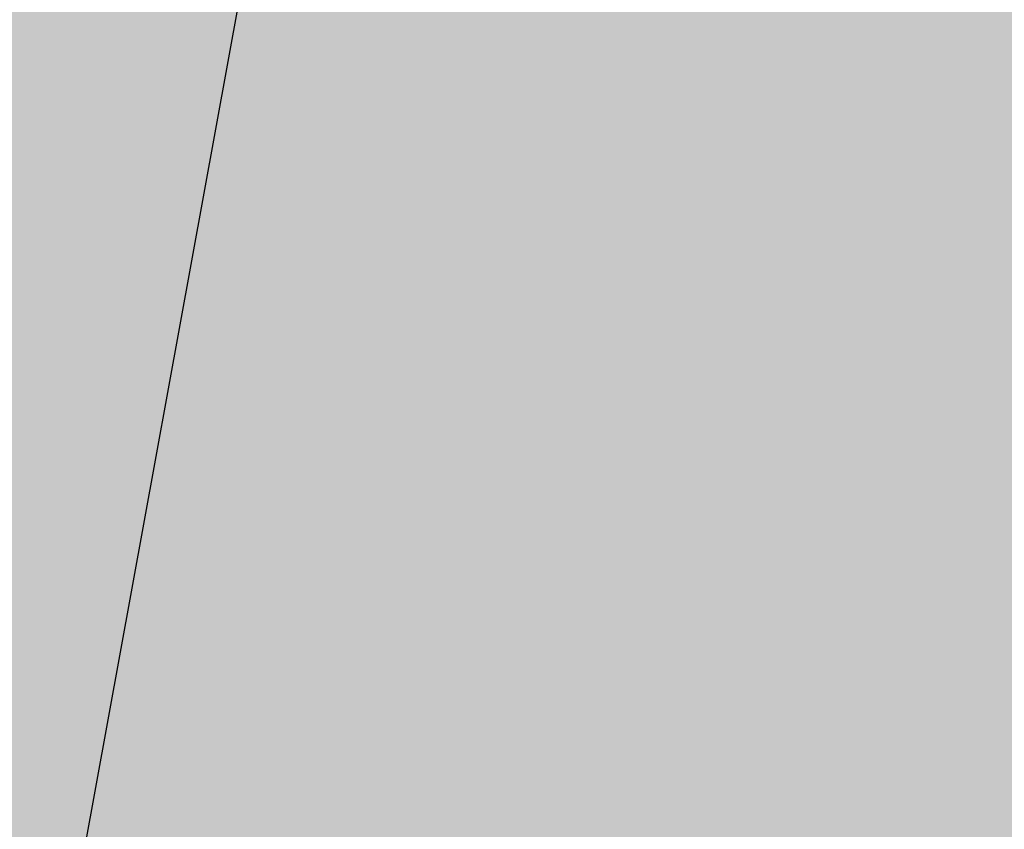
# Model space of a CAD drawing. Units: feet. Extents: x 3168 to 4724, y 827 to 1477.
# Tile 225 of 256: x 3379.08 to 3394.29, y 1074.89 to 1087.4. Entities that reach past the tile are written whole.
import ezdxf

# ---------------------------------------------------------------- set-up
doc = ezdxf.new("R2010")
doc.units = ezdxf.units.FT
doc.layers.add('A-ELEV-PATT', color=8, linetype='Continuous', lineweight=13)
doc.layers.add('C-TOPO', color=3, linetype='Continuous', lineweight=25)

msp = doc.modelspace()

# ---------------------------------------------------------------- hatches: boundary and pattern name
at = {"layer": 'A-ELEV-PATT'}
h = msp.add_hatch(color=256, dxfattribs=at)
h.dxf.hatch_style = 1
edge = h.paths.add_edge_path()
edge.add_ellipse((3552.906, 979.22), major_axis=(36.745, 0), ratio=0.484848, start_angle=0, end_angle=360)
edge = h.paths.add_edge_path()
edge.add_ellipse((3559.892, 929.252), major_axis=(36.745, 0), ratio=0.484848, start_angle=0, end_angle=360)
edge = h.paths.add_edge_path()
edge.add_line((3299.317, 1198.606), (3479.917, 1198.606))
edge.add_line((3479.917, 1198.606), (3479.917, 1209.869))
edge.add_spline(control_points=[(3479.917, 1209.869), (3464.301, 1209.869), (3448.686, 1209.869), (3410.949, 1209.869), (3388.828, 1209.869), (3355.647, 1209.869), (3344.586, 1209.869), (3327.996, 1209.869), (3322.466, 1209.869), (3314.17, 1209.869), (3311.405, 1209.869), (3307.257, 1209.869), (3305.875, 1209.869), (3303.801, 1209.869), (3303.11, 1209.869), (3302.073, 1209.869), (3301.727, 1209.869), (3301.209, 1209.869), (3301.036, 1209.869), (3300.777, 1209.869), (3300.69, 1209.869), (3300.561, 1209.869), (3300.517, 1209.869), (3300.453, 1209.869), (3300.431, 1209.869), (3300.399, 1209.869), (3300.388, 1209.869), (3300.366, 1209.869), (3300.346, 1209.869), (3300.346, 1209.869), (3300.346, 1209.869), (3300.343, 1209.869), (3300.341, 1209.869), (3300.338, 1209.869), (3300.337, 1209.869), (3300.334, 1209.869), (3300.332, 1209.869), (3300.326, 1209.869), (3300.321, 1209.869), (3300.311, 1209.869), (3300.306, 1209.869), (3300.291, 1209.869), (3300.28, 1209.869), (3300.232, 1209.869), (3300.195, 1209.869), (3299.951, 1209.871), (3299.745, 1209.874), (3299.437, 1209.883), (3299.334, 1209.887), (3299.181, 1209.893), (3299.13, 1209.895), (3298.652, 1209.917), (3298.229, 1209.946), (3297.602, 1210.002), (3297.393, 1210.023), (3297.083, 1210.058), (3296.979, 1210.07), (3296.293, 1210.155), (3295.718, 1210.243), (3294.869, 1210.399), (3294.588, 1210.454), (3294.169, 1210.543), (3294.03, 1210.574), (3291.707, 1211.101), (3289.654, 1211.813), (3285.776, 1213.564), (3283.951, 1214.603), (3280.512, 1216.98), (3278.897, 1218.318), (3276.38, 1220.829), (3275.416, 1221.918), (3274.039, 1223.708), (3273.581, 1224.35), (3273.143, 1225.016)], knot_values=[39.119033, 39.119033, 39.119033, 39.119033, 39.286353, 39.286353, 39.523379, 39.523379, 39.641892, 39.641892, 39.701148, 39.701148, 39.730777, 39.730777, 39.745591, 39.745591, 39.752998, 39.752998, 39.756701, 39.756701, 39.758553, 39.758553, 39.759479, 39.759479, 39.759942, 39.759942, 39.760173, 39.760173, 39.760289, 39.760289, 39.760405, 39.760405, 39.760463, 39.760463, 39.763389, 39.763389, 39.764851, 39.764851, 39.767304, 39.767304, 39.773825, 39.773825, 39.78057, 39.78057, 39.79477, 39.79477, 39.845194, 39.845194, 40.126715, 40.126715, 40.267476, 40.267476, 40.337856, 40.337856, 40.927023, 40.927023, 41.221606, 41.221606, 41.368898, 41.368898, 42.202622, 42.202622, 42.619485, 42.619485, 42.827916, 42.827916, 46.118323, 46.118323, 49.408731, 49.408731, 52.699139, 52.699139, 54.927489, 54.927489, 56.104228, 56.104228, 56.104228, 56.104228], weights=[1, 1, 1, 1, 1, 1, 1, 1, 1, 1, 1, 1, 1, 1, 1, 1, 1, 1, 1, 1, 1, 1, 1, 1, 1, 1, 1, 1, 1, 1, 1, 1, 1, 1, 1, 1, 1, 1, 1, 1, 1, 1, 1, 1, 1, 1, 1, 1, 1, 1, 1, 1, 1, 1, 1, 1, 1, 1, 1, 1, 1, 1, 1, 1, 1, 1, 1, 1, 1, 1, 1, 1, 1, 1], degree=3, periodic=0)
edge.add_line((3273.143, 1225.016), (3273.143, 1099.016))
edge.add_line((3273.143, 1099.016), (3299.317, 1099.016))
edge.add_line((3299.317, 1099.016), (3299.317, 1198.606))
edge = h.paths.add_edge_path()
edge.add_line((3304.758, 1324.158), (3479.917, 1324.158))
edge.add_line((3479.917, 1324.158), (3479.917, 1335.715))
edge.add_line((3479.917, 1335.715), (3269.162, 1335.715))
edge.add_spline(control_points=[(3269.162, 1335.715), (3264.024, 1335.715), (3258.364, 1328.958), (3259.264, 1323.9)], knot_values=[0, 0, 0, 0, 15.412191, 15.412191, 15.412191, 15.412191], degree=3, periodic=0)
edge.add_line((3259.264, 1323.9), (3265.517, 1288.769))
edge.add_line((3265.517, 1288.769), (3275.265, 1261.546))
edge.add_line((3275.265, 1261.546), (3304.758, 1261.546))
edge.add_line((3304.758, 1261.546), (3304.758, 1324.158))
h = msp.add_hatch(color=256, dxfattribs=at)
h.dxf.hatch_style = 1
h.paths.add_polyline_path([(3384.525, 1099.016), (3335.029, 1099.016), (3299.317, 1099.016), (3273.143, 1099.016), (3217.565, 1099.016), (3168.069, 827.116), (3335.029, 827.116)])
h = msp.add_hatch(color=256, dxfattribs=at)
h.dxf.hatch_style = 1
h.paths.add_polyline_path([(3845.376, 1099.016), (3706.288, 1099.016), (3715.619, 1081.396), (3715.619, 1052.31), (3792.055, 907.956), (3463.222, 903.642), (3462.899, 928.257, 0.540152), (3462.899, 1014.083), (3621.899, 1014.083), (3601.657, 1052.31), (3601.657, 1081.396), (3592.327, 1099.016), (3384.525, 1099.016), (3335.029, 827.116), (3845.376, 827.116)])

# ---------------------------------------------------------------- linework, layer by layer
at = {"layer": 'C-TOPO'}
msp.add_line((3384.525, 1099.016), (3335.029, 827.116), dxfattribs=at)
msp.add_lwpolyline([(3384.525, 1099.016), (3335.029, 827.116), (3845.376, 827.116), (3845.376, 1099.016), (3335.029, 1099.016)], dxfattribs=at)

doc.saveas('drawing.dxf')
